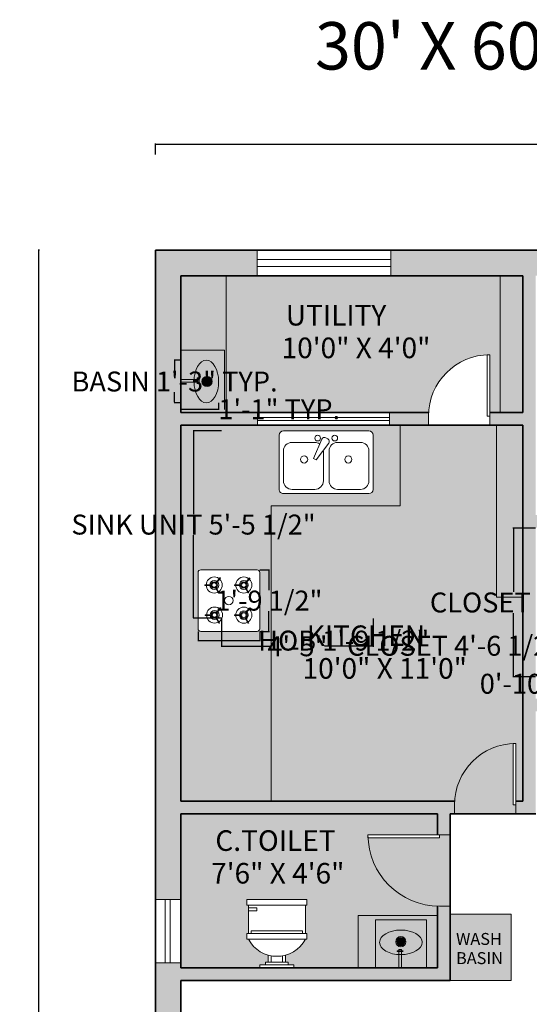
# Model space of a CAD drawing. Units: inches. Extents: x 2167 to 2589, y 1680 to 2489.
# Tile 35 of 38: x 2167 to 2346, y 2143 to 2489. Entities that reach past the tile are written whole.
import ezdxf

# ---------------------------------------------------------------- set-up
doc = ezdxf.new("R2010")
doc.units = ezdxf.units.IN
doc.header["$MEASUREMENT"] = 0
doc.layers.get('0').update_dxf_attribs({"color": 250})
for name, color, linetype, lineweight in [('A-ANNO-DIMS', 2, 'Continuous', 18), ('A-AREA-IDEN', 7, 'Continuous', 18), ('A-DOOR', 4, 'Continuous', 18), ('A-EQPM', 34, 'Continuous', 18), ('A-FLOR-FIXT', 8, 'Continuous', 18), ('A-FURN-FIXD', 34, 'Continuous', 18), ('A-WALL-PATT', 250, 'Continuous', 13), ('C-PROP', 7, 'Continuous', 35), ('furniture', 34, 'Continuous', 18), ('text', 7, 'Continuous', 25), ('walls', 7, 'Continuous', 35), ('windows', 141, 'Continuous', 18)]:
    doc.layers.add(name, color=color, linetype=linetype, lineweight=lineweight)
for name, color, linetype, lineweight, true_color in [('A-FLOR-FIXT-PATT', 7, 'Continuous', 13, 0xebebeb), ('A-FLOR-PATT', 254, 'Continuous', 13, 0xfeeab9), ('A-FURN-FIXD-PATT', 33, 'Continuous', 13, 0xcd8e5c)]:
    doc.layers.add(name, color=color, linetype=linetype, lineweight=lineweight, true_color=true_color)
doc.styles.add('ATT', font='TXT')
doc.styles.get("Standard").update_dxf_attribs({"font": 'arial.ttf'})
doc.dimstyles.get("Standard").update_dxf_attribs({"dimtxt": 7, "dimasz": 0.18, "dimexe": 0.18, "dimexo": 0.0625, "dimgap": 0.09, "dimtad": 0, "dimtih": 1, "dimtoh": 1, "dimdec": 1, "dimzin": 0, "dimdsep": 46, "dimlunit": 3, "dimtxsty": 'Standard', "dimcen": 0.09, "dimadec": 0, "dimazin": 0, "dimtfac": 1, "dimtdec": 1, "dimtofl": 0, "dimtmove": 0, "dimatfit": 3, "dimfxl": 1, "dimtolj": 1, "dimtzin": 0, "dimarcsym": 0})

# ---------------------------------------------------------------- blocks, each defined once
blk = doc.blocks.new('*U2')
for p, q in [((0, 0), (0, -6)), ((40, 0), (40, -6))]:
    blk.add_line(p, q)
blk.add_lwpolyline([(0, 0), (0, 40), (1.75, 40), (1.75, 0)], close=True)
blk.add_arc((0, 0), 40, 0, 90)
blk = doc.blocks.new('4bstove')
at = {"layer": 'furniture'}
for p, q in [((1452.73, 1446.21), (1452.73, 1448.61)), ((1452.98, 1446.22), (1452.98, 1448.61)), ((1464.44, 1446.34), (1464.44, 1448.73)), ((1464.69, 1446.34), (1464.69, 1448.73)), ((1463.45, 1444.58), (1461.38, 1443.38)), ((1451.74, 1444.45), (1449.67, 1443.25)), ((1451.87, 1444.23), (1449.79, 1443.04)), ((1453.75, 1444.08), (1455.58, 1442.54)), ((1453.91, 1444.27), (1455.74, 1442.73)), ((1463.57, 1444.36), (1461.5, 1443.17)), ((1465.46, 1444.21), (1467.29, 1442.67)), ((1465.62, 1444.4), (1467.45, 1442.86)), ((1452.69, 1434.81), (1452.69, 1437.2)), ((1452.94, 1434.81), (1452.94, 1437.2)), ((1464.44, 1434.81), (1464.44, 1437.2)), ((1464.69, 1434.81), (1464.69, 1437.2)), ((1451.7, 1433.04), (1449.63, 1431.85)), ((1463.45, 1433.04), (1461.38, 1431.85)), ((1451.82, 1432.83), (1449.75, 1431.63)), ((1453.71, 1432.67), (1455.54, 1431.13)), ((1453.87, 1432.86), (1455.7, 1431.33)), ((1463.57, 1432.83), (1461.5, 1431.63)), ((1465.46, 1432.67), (1467.29, 1431.13)), ((1465.62, 1432.86), (1467.45, 1431.33))]:
    blk.add_line(p, q, dxfattribs=at)
for points in [[(1447.5, 1427.38), (1469.5, 1427.38, 0.414214), (1470.5, 1428.38), (1470.5, 1450.38, 0.414214), (1469.5, 1451.38), (1447.5, 1451.38, 0.414214), (1446.5, 1450.38), (1446.5, 1428.38, 0.414214)], [(1453.75, 1444.97, 1), (1452, 1444.97, 1)], [(1465.46, 1445.1, 1), (1463.71, 1445.1, 1)], [(1453.71, 1433.56, 1), (1451.96, 1433.56, 1)], [(1465.46, 1433.56, 1), (1463.71, 1433.56, 1)]]:
    blk.add_lwpolyline(points, format="xyb", close=True, dxfattribs=at)
for points in [[(1454.12, 1444.97, 1), (1451.62, 1444.97, 1), (1454.12, 1444.97, 1)], [(1465.83, 1445.1, 1), (1463.33, 1445.1, 1), (1465.83, 1445.1, 1)], [(1454.08, 1433.56, 1), (1451.58, 1433.56, 1), (1454.08, 1433.56, 1)], [(1465.83, 1433.56, 1), (1463.33, 1433.56, 1), (1465.83, 1433.56, 1)]]:
    blk.add_lwpolyline(points, format="xyb", dxfattribs=at)
for centre, radius in [((1452.87, 1444.97), 3.14), ((1452.87, 1444.97), 1.75), ((1464.58, 1445.1), 3.14), ((1464.58, 1445.1), 1.75), ((1458.5, 1439.38), 1.67), ((1452.83, 1433.56), 3.14), ((1452.83, 1433.56), 1.75), ((1464.58, 1433.56), 3.14), ((1464.58, 1433.56), 1.75)]:
    blk.add_circle(centre, radius, dxfattribs=at)
for centre, start, end in [((1452.87, 1444.97), 88.2645, 92.2039), ((1464.58, 1445.1), 88.2645, 92.2039), ((1452.87, 1444.97), 208.188, 212.1274), ((1452.87, 1444.97), 318.1018, 322.0412), ((1464.58, 1445.1), 208.188, 212.1274), ((1464.58, 1445.1), 318.1018, 322.0412), ((1452.83, 1433.56), 88.2645, 92.2039), ((1464.58, 1433.56), 88.2645, 92.2039)]:
    blk.add_arc(centre, 3.64, start, end, dxfattribs=at)
blk = doc.blocks.new('stove')
at = {"layer": 'furniture', "xscale": 0.9, "yscale": 0.9, "zscale": 0.9, "rotation": 89.99999999999999}
blk.add_blockref('4bstove', (1295.44, -1312.65), dxfattribs=at)
blk = doc.blocks.new('15PSNK10')
at = {"color": 0, "linetype": 'ByBlock'}
for p, q in [((0, 15), (0, -15)), ((20.5, 16.5), (1.5, 16.5)), ((7, 15), (17.5, 15)), ((22, -15), (22, 15)), ((4, 4), (4, 12)), ((20.5, 12), (20.5, 4)), ((2.37, -0.1), (2.77, 0.6)), ((10.18, -3.57), (4.27, 0.87)), ((17.5, 1), (7, 1)), ((2.88, -1.54), (9.68, -4.43)), ((7.04, -1), (17.5, -1)), ((4, -12), (4, -4)), ((9.68, -4.43), (10.18, -3.57)), ((20.5, -4), (20.5, -12)), ((1.5, -16.5), (20.5, -16.5)), ((17.5, -15), (7, -15))]:
    blk.add_line(p, q, dxfattribs=at)
for centre, radius in [((10, 7.75), 1.25), ((2.5, 3), 1), ((2.5, -3), 1), ((10, -7.75), 1.25)]:
    blk.add_circle(centre, radius, dxfattribs=at)
for centre, radius, start, end in [((1.5, 15), 1.5, 90, 180), ((7, 12), 3, 90, 180), ((17.5, 12), 3, 0, 90), ((20.5, 15), 1.5, 0, 90), ((7, 4), 3, 180, 270), ((17.5, 4), 3, 270, 0), ((3.63, 0.1), 1, 50.5377, 150), ((3.23, -0.6), 1, 150, 249.4623), ((7, -4), 3, 146.607, 180), ((17.5, -4), 3, 0, 90), ((7, -12), 3, 180, 270), ((17.5, -12), 3, 270, 0), ((1.5, -15), 1.5, 180, 270), ((20.5, -15), 1.5, 270, 0)]:
    blk.add_arc(centre, radius, start, end, dxfattribs=at)
at = {"color": 0, "linetype": 'ByBlock', "style": 'ATT'}
for tag, p, flags in [('ITEM', (0, -26), 3), ('ROOM_NUMBER', (0, -35), 1)]:
    blk.add_attdef(tag, p, '', height=6, dxfattribs=dict(at, flags=flags))
blk = doc.blocks.new('*U11')
for p, q in [((-10, 22), (-10, 12)), ((-10, 21), (-7, 21)), ((-7, 21), (-7, 20)), ((10, 12), (10, 22)), ((-7, 20), (-10, 20)), ((10.5, 12), (-10.5, 12)), ((-10.5, 10), (-10.5, 12)), ((9, 13), (-9, 13)), ((-9, 13), (-9, 12)), ((9, 12), (9, 13)), ((10.5, 12), (10.5, 10)), ((10.5, 10), (-10.5, 10)), ((-3, 4.4065), (-3, 2)), ((-2, 2), (-2, 4.1658)), ((2, 4.1658), (2, 2)), ((3, 2), (3, 4.4065)), ((4, 2), (-4, 2)), ((-4, 2), (-4, 1)), ((4, 1), (4, 2))]:
    blk.add_line(p, q)
for points in [[(10.5, 22), (10.5, 24), (-10.5, 24), (-10.5, 22)], [(6, 0), (6, 1), (-6, 1), (-6, 0)]]:
    blk.add_lwpolyline(points, close=True)
blk.add_arc((0, 15.3333), 11.3333, 208.0725, 331.9275)
blk = doc.blocks.new('*D23')
at = {"layer": 'A-ANNO-DIMS', "color": 0, "lineweight": -2, "transparency": 16777216}
for p, q in [((2215.05, 2441.31), (2215.05, 2445.11)), ((2215.23, 2444.93), (2389.02, 2444.93)), ((2574.87, 2444.93), (2401.08, 2444.93)), ((2575.05, 2441.31), (2575.05, 2445.11))]:
    blk.add_line(p, q, dxfattribs=at)
at = {"layer": 'A-ANNO-DIMS', "color": 0, "transparency": 16777216}
for points in [[(2215.23, 2444.96), (2215.23, 2444.9), (2215.05, 2444.93)], [(2574.87, 2444.96), (2574.87, 2444.9), (2575.05, 2444.93)]]:
    blk.add_solid(points, dxfattribs=at)
at = {"layer": 'Defpoints', "color": 0, "transparency": 16777216}
for p in [(2575.05, 2444.93), (2215.05, 2441.25), (2575.05, 2441.25)]:
    blk.add_point(p, dxfattribs=at)
at = {"layer": 'A-ANNO-DIMS', "color": 0, "transparency": 16777216, "insert": (2395.05, 2444.93), "char_height": 7, "attachment_point": 5}
blk.add_mtext("\\A1;30'", dxfattribs=at)
blk = doc.blocks.new('*D24')
at = {"layer": 'A-ANNO-DIMS', "color": 0, "lineweight": -2, "transparency": 16777216}
for p, q in [((2174.43, 2407.69), (2173.89, 2407.69)), ((2174.07, 2407.51), (2174.07, 2051.36)), ((2174.07, 1687.87), (2174.07, 2044.03)), ((2174.43, 1687.69), (2173.89, 1687.69))]:
    blk.add_line(p, q, dxfattribs=at)
at = {"layer": 'A-ANNO-DIMS', "color": 0, "transparency": 16777216}
for points in [[(2174.04, 2407.51), (2174.1, 2407.51), (2174.07, 2407.69)], [(2174.04, 1687.87), (2174.1, 1687.87), (2174.07, 1687.69)]]:
    blk.add_solid(points, dxfattribs=at)
at = {"layer": 'Defpoints', "color": 0, "transparency": 16777216}
for p in [(2174.49, 2407.69), (2174.07, 1687.69), (2174.49, 1687.69)]:
    blk.add_point(p, dxfattribs=at)
at = {"layer": 'A-ANNO-DIMS', "color": 0, "transparency": 16777216, "insert": (2174.07, 2047.69), "char_height": 7, "attachment_point": 5}
blk.add_mtext("\\A1;60'", dxfattribs=at)
blk = doc.blocks.new('LAV-OVAL-WITH-TAP')
for p, q in [((6.14, 5.63), (6.14, 5.92)), ((6.14, 5.92), (8.26, 5.92)), ((8.26, 5.63), (6.14, 5.63)), ((7.69, 6.42), (6.74, 6.42)), ((6.74, 6.42), (6.74, 0)), ((7.69, 6.42), (7.69, 0))]:
    blk.add_line(p, q)
for radius in [1.79, 1.79, 1.43, 1.43, 1.43, 1.43]:
    blk.add_circle((7.46, 9.13), radius)
blk.add_ellipse((7.48, 8.9), major_axis=(7.48, 0.02), ratio=0.576535)
blk = doc.blocks.new('*D31')
at = {"layer": 'A-ANNO-DIMS', "color": 0, "lineweight": -2, "transparency": 16777216}
for p, q in [((2223.99, 2369.03), (2221.62, 2369.03)), ((2221.8, 2368.85), (2221.8, 2365.26)), ((2221.8, 2354.24), (2221.8, 2357.83)), ((2223.99, 2354.06), (2221.62, 2354.06))]:
    blk.add_line(p, q, dxfattribs=at)
at = {"layer": 'A-ANNO-DIMS', "color": 0, "transparency": 16777216}
for points in [[(2221.77, 2368.85), (2221.83, 2368.85), (2221.8, 2369.03)], [(2221.77, 2354.24), (2221.83, 2354.24), (2221.8, 2354.06)]]:
    blk.add_solid(points, dxfattribs=at)
at = {"layer": 'Defpoints', "color": 0, "transparency": 16777216}
for p in [(2224.05, 2369.03), (2221.8, 2354.06), (2224.05, 2354.06)]:
    blk.add_point(p, dxfattribs=at)
at = {"layer": 'A-ANNO-DIMS', "color": 0, "transparency": 16777216, "insert": (2221.8, 2361.54), "char_height": 7, "attachment_point": 5}
blk.add_mtext('\\A1;BASIN 1\'-3" TYP.', dxfattribs=at)
blk = doc.blocks.new('*D32')
at = {"layer": 'A-ANNO-DIMS', "color": 0, "lineweight": -2, "transparency": 16777216}
for p, q in [((2224.05, 2354), (2224.05, 2351.63)), ((2224.23, 2351.81), (2237.09, 2351.81)), ((2237.27, 2354), (2237.27, 2351.63)), ((2237.27, 2351.81), (2237.45, 2351.81))]:
    blk.add_line(p, q, dxfattribs=at)
at = {"layer": 'A-ANNO-DIMS', "color": 0, "transparency": 16777216}
for points in [[(2224.23, 2351.84), (2224.23, 2351.78), (2224.05, 2351.81)], [(2237.09, 2351.84), (2237.09, 2351.78), (2237.27, 2351.81)]]:
    blk.add_solid(points, dxfattribs=at)
at = {"layer": 'Defpoints', "color": 0, "transparency": 16777216}
for p in [(2224.05, 2354.06), (2237.27, 2354.06), (2237.27, 2351.81)]:
    blk.add_point(p, dxfattribs=at)
at = {"layer": 'A-ANNO-DIMS', "color": 0, "transparency": 16777216, "insert": (2258.54, 2351.81), "char_height": 7, "attachment_point": 5}
blk.add_mtext('\\A1;1\'-1" TYP.', dxfattribs=at)
blk = doc.blocks.new('*D33')
at = {"layer": 'A-ANNO-DIMS', "color": 0, "lineweight": -2, "transparency": 16777216}
for p, q in [((2358.53, 2268.74), (2358.35, 2268.74)), ((2358.53, 2260.62), (2358.53, 2268.92)), ((2412.91, 2268.74), (2358.71, 2268.74)), ((2413.09, 2260.62), (2413.09, 2268.92))]:
    blk.add_line(p, q, dxfattribs=at)
at = {"layer": 'A-ANNO-DIMS', "color": 0, "transparency": 16777216}
for points in [[(2358.71, 2268.77), (2358.71, 2268.71), (2358.53, 2268.74)], [(2412.91, 2268.77), (2412.91, 2268.71), (2413.09, 2268.74)]]:
    blk.add_solid(points, dxfattribs=at)
at = {"layer": 'Defpoints', "color": 0, "transparency": 16777216}
for p in [(2358.53, 2268.74), (2358.53, 2260.56), (2413.09, 2260.56)]:
    blk.add_point(p, dxfattribs=at)
at = {"layer": 'A-ANNO-DIMS', "color": 0, "transparency": 16777216, "insert": (2319.92, 2268.74), "char_height": 7, "attachment_point": 5}
blk.add_mtext('\\A1;CLOSET 4\'-6 1/2"', dxfattribs=at)
blk = doc.blocks.new('*D34')
at = {"layer": 'A-ANNO-DIMS', "color": 0, "lineweight": -2, "transparency": 16777216}
for p, q in [((2358.47, 2260.56), (2350.17, 2260.56)), ((2350.35, 2260.38), (2350.35, 2259.11)), ((2350.35, 2250.42), (2350.35, 2251.69)), ((2358.47, 2250.24), (2350.17, 2250.24))]:
    blk.add_line(p, q, dxfattribs=at)
at = {"layer": 'A-ANNO-DIMS', "color": 0, "transparency": 16777216}
for points in [[(2350.32, 2260.38), (2350.38, 2260.38), (2350.35, 2260.56)], [(2350.32, 2250.42), (2350.38, 2250.42), (2350.35, 2250.24)]]:
    blk.add_solid(points, dxfattribs=at)
at = {"layer": 'Defpoints', "color": 0, "transparency": 16777216}
for p in [(2358.53, 2260.56), (2350.35, 2250.24), (2358.53, 2250.24)]:
    blk.add_point(p, dxfattribs=at)
at = {"layer": 'A-ANNO-DIMS', "color": 0, "transparency": 16777216, "insert": (2350.35, 2255.4), "char_height": 7, "attachment_point": 5}
blk.add_mtext('\\A1;0\'-10 1/2"', dxfattribs=at)
blk = doc.blocks.new('*D37')
at = {"layer": 'A-ANNO-DIMS', "color": 0, "lineweight": -2, "transparency": 16777216}
for p, q in [((2348.49, 2310.05), (2340.54, 2310.05)), ((2340.72, 2309.87), (2340.72, 2287.66)), ((2340.72, 2258.02), (2340.72, 2280.23)), ((2348.49, 2257.84), (2340.54, 2257.84))]:
    blk.add_line(p, q, dxfattribs=at)
at = {"layer": 'A-ANNO-DIMS', "color": 0, "transparency": 16777216}
for points in [[(2340.69, 2309.87), (2340.75, 2309.87), (2340.72, 2310.05)], [(2340.69, 2258.02), (2340.75, 2258.02), (2340.72, 2257.84)]]:
    blk.add_solid(points, dxfattribs=at)
at = {"layer": 'Defpoints', "color": 0, "transparency": 16777216}
for p in [(2348.55, 2310.05), (2340.72, 2257.84), (2348.55, 2257.84)]:
    blk.add_point(p, dxfattribs=at)
at = {"layer": 'A-ANNO-DIMS', "color": 0, "transparency": 16777216, "insert": (2340.72, 2283.95), "char_height": 7, "attachment_point": 5}
blk.add_mtext('\\A1;CLOSET 4\'-4"', dxfattribs=at)
blk = doc.blocks.new('*D49')
at = {"layer": 'A-ANNO-DIMS', "color": 0, "lineweight": -2, "transparency": 16777216}
for p, q in [((2230.07, 2273.74), (2230.07, 2270.38)), ((2251.67, 2273.74), (2251.67, 2270.38)), ((2230.25, 2270.56), (2251.49, 2270.56)), ((2251.67, 2270.56), (2251.85, 2270.56))]:
    blk.add_line(p, q, dxfattribs=at)
at = {"layer": 'A-ANNO-DIMS', "color": 0, "transparency": 16777216}
for points in [[(2230.25, 2270.59), (2230.25, 2270.53), (2230.07, 2270.56)], [(2251.49, 2270.59), (2251.49, 2270.53), (2251.67, 2270.56)]]:
    blk.add_solid(points, dxfattribs=at)
at = {"layer": 'Defpoints', "color": 0, "transparency": 16777216}
for p in [(2230.07, 2273.8), (2251.67, 2273.8), (2251.67, 2270.56)]:
    blk.add_point(p, dxfattribs=at)
at = {"layer": 'A-ANNO-DIMS', "color": 0, "transparency": 16777216, "insert": (2281.17, 2270.56), "char_height": 7, "attachment_point": 5}
blk.add_mtext('\\A1;HOB 1\'-9 1/2"', dxfattribs=at)
blk = doc.blocks.new('*D50')
at = {"layer": 'A-ANNO-DIMS', "color": 0, "lineweight": -2, "transparency": 16777216}
for p, q in [((2251.74, 2295.4), (2255.09, 2295.4)), ((2254.91, 2295.22), (2254.91, 2288.31)), ((2254.91, 2273.98), (2254.91, 2280.89)), ((2251.74, 2273.8), (2255.09, 2273.8))]:
    blk.add_line(p, q, dxfattribs=at)
at = {"layer": 'A-ANNO-DIMS', "color": 0, "transparency": 16777216}
for points in [[(2254.88, 2295.22), (2254.94, 2295.22), (2254.91, 2295.4)], [(2254.88, 2273.98), (2254.94, 2273.98), (2254.91, 2273.8)]]:
    blk.add_solid(points, dxfattribs=at)
at = {"layer": 'Defpoints', "color": 0, "transparency": 16777216}
for p in [(2251.67, 2295.4), (2254.91, 2295.4), (2251.67, 2273.8)]:
    blk.add_point(p, dxfattribs=at)
at = {"layer": 'A-ANNO-DIMS', "color": 0, "transparency": 16777216, "insert": (2254.91, 2284.6), "char_height": 7, "attachment_point": 5}
blk.add_mtext('\\A1;1\'-9 1/2"', dxfattribs=at)
blk = doc.blocks.new('*D53')
at = {"layer": 'A-ANNO-DIMS', "color": 0, "lineweight": -2, "transparency": 16777216}
for p, q in [((2238.25, 2344.17), (2228.27, 2344.17)), ((2228.45, 2343.99), (2228.45, 2315.01)), ((2228.45, 2278.61), (2228.45, 2307.59)), ((2238.25, 2278.43), (2228.27, 2278.43))]:
    blk.add_line(p, q, dxfattribs=at)
at = {"layer": 'A-ANNO-DIMS', "color": 0, "transparency": 16777216}
for points in [[(2228.42, 2343.99), (2228.48, 2343.99), (2228.45, 2344.17)], [(2228.42, 2278.61), (2228.48, 2278.61), (2228.45, 2278.43)]]:
    blk.add_solid(points, dxfattribs=at)
at = {"layer": 'Defpoints', "color": 0, "transparency": 16777216}
for p in [(2238.31, 2344.17), (2228.45, 2278.43), (2238.31, 2278.43)]:
    blk.add_point(p, dxfattribs=at)
at = {"layer": 'A-ANNO-DIMS', "color": 0, "transparency": 16777216, "insert": (2228.45, 2311.3), "char_height": 7, "attachment_point": 5}
blk.add_mtext('\\A1;SINK UNIT 5\'-5 1/2"', dxfattribs=at)
blk = doc.blocks.new('*D54')
at = {"layer": 'A-ANNO-DIMS', "color": 0, "lineweight": -2, "transparency": 16777216}
for p, q in [((2238.31, 2278.36), (2238.31, 2268.39)), ((2291.52, 2278.36), (2291.52, 2268.39)), ((2238.49, 2268.57), (2255.38, 2268.57)), ((2291.34, 2268.57), (2274.45, 2268.57))]:
    blk.add_line(p, q, dxfattribs=at)
at = {"layer": 'A-ANNO-DIMS', "color": 0, "transparency": 16777216}
for points in [[(2238.49, 2268.6), (2238.49, 2268.54), (2238.31, 2268.57)], [(2291.34, 2268.6), (2291.34, 2268.54), (2291.52, 2268.57)]]:
    blk.add_solid(points, dxfattribs=at)
at = {"layer": 'Defpoints', "color": 0, "transparency": 16777216}
for p in [(2238.31, 2278.43), (2291.52, 2278.43), (2291.52, 2268.57)]:
    blk.add_point(p, dxfattribs=at)
at = {"layer": 'A-ANNO-DIMS', "color": 0, "transparency": 16777216, "insert": (2264.92, 2268.57), "char_height": 7, "attachment_point": 5}
blk.add_mtext('\\A1;4\'-5"', dxfattribs=at)

msp = doc.modelspace()

# ---------------------------------------------------------------- hatches: boundary and pattern name
at = {"layer": 'A-FLOR-FIXT-PATT'}
h = msp.add_hatch(color=256, dxfattribs=at)
h.dxf.hatch_style = 1
edge = h.paths.add_edge_path()
edge.add_line((2239.3, 2351.68), (2239.3, 2372.58))
edge.add_line((2239.3, 2372.58), (2224.05, 2372.58))
edge.add_line((2224.05, 2372.58), (2224.05, 2362.28))
edge.add_line((2224.05, 2362.28), (2228.65, 2362.28))
edge.add_ellipse((2232.94, 2361.54), major_axis=(0.02, -7.48), ratio=0.576535, start_angle=272.6137, end_angle=620.1108, ccw=False)
edge.add_line((2228.63, 2361.34), (2224.05, 2361.34))
edge.add_line((2224.05, 2361.34), (2224.05, 2351.68))
edge.add_line((2224.05, 2351.68), (2239.3, 2351.68))
h = msp.add_hatch(color=256, dxfattribs=at)
h.dxf.hatch_style = 1
edge = h.paths.add_edge_path()
edge.add_ellipse((2232.94, 2361.54), major_axis=(0.02, -7.48), ratio=0.576535, start_angle=272.6137, end_angle=260.1108)
edge.add_line((2228.65, 2362.28), (2229.68, 2362.28))
edge.add_line((2229.68, 2362.28), (2229.68, 2362.88))
edge.add_line((2229.68, 2362.88), (2229.97, 2362.88))
edge.add_line((2229.97, 2362.88), (2229.97, 2362.28))
edge.add_line((2229.97, 2362.28), (2230.47, 2362.28))
edge.add_line((2230.47, 2362.28), (2230.47, 2361.34))
edge.add_line((2230.47, 2361.34), (2228.63, 2361.34))
h.paths.add_polyline_path([(2233.18, 2359.77, -1), (2233.18, 2363.35, -1)], flags=16)
h.paths.add_polyline_path([(2233.18, 2362.99, -1), (2233.18, 2360.13, -1)], flags=0)
h.paths.add_polyline_path([(2233.18, 2360.13, 1), (2233.18, 2362.99, 1)], flags=0)
edge = h.paths.add_edge_path()
edge.add_line((2229.68, 2361.34), (2229.68, 2362.28))
edge.add_line((2229.68, 2362.28), (2228.65, 2362.28))
edge.add_ellipse((2232.94, 2361.54), major_axis=(0.02, -7.48), ratio=0.576535, start_angle=260.1108, end_angle=272.6137)
edge.add_line((2228.63, 2361.34), (2229.68, 2361.34))
h.paths.add_polyline_path([(2230.47, 2361.34), (2230.47, 2362.28), (2229.97, 2362.28), (2229.97, 2361.34)], flags=17)
h.paths.add_polyline_path([(2229.97, 2361.34), (2229.97, 2362.28), (2229.68, 2362.28), (2229.68, 2361.34)], flags=17)
h.paths.add_polyline_path([(2229.97, 2362.28), (2229.97, 2362.88), (2229.68, 2362.88), (2229.68, 2362.28)], flags=17)
edge = h.paths.add_edge_path()
edge.add_ellipse((2232.94, 2361.54), major_axis=(0.02, -7.48), ratio=0.576535, start_angle=260.1108, end_angle=272.6137, ccw=False)
edge.add_line((2228.65, 2362.28), (2224.05, 2362.28))
edge.add_line((2224.05, 2362.28), (2224.05, 2361.34))
edge.add_line((2224.05, 2361.34), (2228.63, 2361.34))
h = msp.add_hatch(color=256, dxfattribs=at)
h.dxf.hatch_style = 1
h.paths.add_polyline_path([(2233.18, 2362.99, 1), (2233.18, 2360.13, 1)], flags=0)
h.paths.add_polyline_path([(2233.18, 2363.35, 1), (2233.18, 2359.77, 1)])
h.paths.add_polyline_path([(2233.18, 2362.99, -1), (2233.18, 2360.13, -1)], flags=16)
h = msp.add_hatch(color=256, dxfattribs=at)
h.dxf.hatch_style = 1
h.paths.add_polyline_path([(2233.18, 2362.99, 1), (2233.18, 2360.13, 1)])
h = msp.add_hatch(color=256, dxfattribs=at)
h.dxf.hatch_style = 1
edge = h.paths.add_edge_path()
edge.add_line((2310.18, 2172.5), (2292.31, 2172.5))
edge.add_line((2292.31, 2172.5), (2292.31, 2155.69))
edge.add_line((2292.31, 2155.69), (2300.49, 2155.69))
edge.add_line((2300.49, 2155.69), (2300.49, 2160.3))
edge.add_ellipse((2301.23, 2164.59), major_axis=(7.48, 0.02), ratio=0.576535, start_angle=272.6137, end_angle=620.1108, ccw=False)
edge.add_line((2301.44, 2160.28), (2301.44, 2155.69))
edge.add_line((2301.44, 2155.69), (2310.18, 2155.69))
edge.add_line((2310.18, 2155.69), (2310.18, 2172.5))
h = msp.add_hatch(color=256, dxfattribs=at)
h.dxf.hatch_style = 1
edge = h.paths.add_edge_path()
edge.add_ellipse((2301.23, 2164.59), major_axis=(7.48, 0.02), ratio=0.576535, start_angle=272.6137, end_angle=260.1108)
edge.add_line((2300.49, 2160.3), (2300.49, 2161.32))
edge.add_line((2300.49, 2161.32), (2299.89, 2161.32))
edge.add_line((2299.89, 2161.32), (2299.89, 2161.62))
edge.add_line((2299.89, 2161.62), (2300.49, 2161.62))
edge.add_line((2300.49, 2161.62), (2300.49, 2162.11))
edge.add_line((2300.49, 2162.11), (2301.44, 2162.11))
edge.add_line((2301.44, 2162.11), (2301.44, 2160.28))
h.paths.add_polyline_path([(2303, 2164.83, -1), (2299.43, 2164.83, -1)], flags=16)
h.paths.add_polyline_path([(2299.79, 2164.83, -1), (2302.64, 2164.83, -1)], flags=0)
edge = h.paths.add_edge_path()
edge.add_ellipse((2301.23, 2164.59), major_axis=(7.48, 0.02), ratio=0.576535, start_angle=260.1108, end_angle=272.6137, ccw=False)
edge.add_line((2300.49, 2160.3), (2300.49, 2155.69))
edge.add_line((2300.49, 2155.69), (2301.44, 2155.69))
edge.add_line((2301.44, 2155.69), (2301.44, 2160.28))
edge = h.paths.add_edge_path()
edge.add_line((2301.44, 2161.32), (2300.49, 2161.32))
edge.add_line((2300.49, 2161.32), (2300.49, 2160.3))
edge.add_ellipse((2301.23, 2164.59), major_axis=(7.48, 0.02), ratio=0.576535, start_angle=260.1108, end_angle=272.6137)
edge.add_line((2301.44, 2160.28), (2301.44, 2161.32))
h.paths.add_polyline_path([(2301.44, 2162.11), (2300.49, 2162.11), (2300.49, 2161.62), (2301.44, 2161.62)], flags=17)
h.paths.add_polyline_path([(2301.44, 2161.62), (2300.49, 2161.62), (2300.49, 2161.32), (2301.44, 2161.32)], flags=17)
h.paths.add_polyline_path([(2300.49, 2161.62), (2299.89, 2161.62), (2299.89, 2161.32), (2300.49, 2161.32)], flags=17)
h = msp.add_hatch(color=256, dxfattribs=at)
h.dxf.hatch_style = 1
h.paths.add_polyline_path([(2302.64, 2164.83, 1), (2299.79, 2164.83, 1)])
at = {"layer": 'A-FLOR-PATT'}
h = msp.add_hatch(color=256, dxfattribs=at)
h.dxf.hatch_style = 1
h.paths.add_polyline_path([(2331.51, 2370.93), (2331.51, 2370.95), (2332.45, 2370.95), (2332.45, 2350.69), (2336.06, 2350.69), (2336.06, 2398.69), (2239.96, 2398.69), (2239.96, 2373.2), (2239.96, 2350.69), (2310.96, 2350.69, -0.38441)])
h = msp.add_hatch(color=256, dxfattribs=at)
h.dxf.hatch_style = 1
h.paths.add_polyline_path([(2289.71, 2201.31), (2289.68, 2201.31), (2289.68, 2202.4), (2314.05, 2202.4), (2314.05, 2209.69), (2224.05, 2209.69), (2224.05, 2155.69), (2251.7, 2155.69), (2251.7, 2156.69), (2253.7, 2156.69), (2253.7, 2157.69), (2254.7, 2157.69), (2254.7, 2160.1, -0.206081), (2247.7, 2165.69), (2247.2, 2165.69), (2247.2, 2167.69), (2247.7, 2167.69), (2247.7, 2177.69), (2247.2, 2177.69), (2247.2, 2179.69), (2268.2, 2179.69), (2268.2, 2177.69), (2267.7, 2177.69), (2267.7, 2167.69), (2268.2, 2167.69), (2268.2, 2165.69), (2267.7, 2165.69, -0.206081), (2260.7, 2160.1), (2260.7, 2157.69), (2261.7, 2157.69), (2261.7, 2156.69), (2263.7, 2156.69), (2263.7, 2155.69), (2286.21, 2155.69), (2286.21, 2173.97), (2314.05, 2173.97), (2314.05, 2177.32, -0.392973)])
h.paths.add_polyline_path([(2318.55, 2202.4), (2314.78, 2202.4), (2314.78, 2201.31), (2289.71, 2201.31, 0.401453), (2314.78, 2177.3), (2318.55, 2177.3)])
h.paths.add_polyline_path([(2344.05, 2285.87), (2334.79, 2285.87), (2334.79, 2346.19), (2300.97, 2346.19), (2300.97, 2317.9), (2255.65, 2317.9), (2255.65, 2214.19), (2320.1, 2214.19, -0.38441), (2340.65, 2234.43), (2340.65, 2234.45), (2341.59, 2234.45), (2341.59, 2214.19), (2344.05, 2214.19)])
h.paths.add_polyline_path([(2340.65, 2234.43, 0.401453), (2320.06, 2212.92), (2320.06, 2209.69), (2341.59, 2209.69), (2341.59, 2212.92), (2340.65, 2212.92)])
at = {"layer": 'A-FURN-FIXD-PATT'}
h = msp.add_hatch(color=256, dxfattribs=at)
h.dxf.hatch_style = 1
h.paths.add_polyline_path([(2239.96, 2398.69), (2224.05, 2398.69), (2224.05, 2373.2), (2239.96, 2373.2)])
h = msp.add_hatch(color=256, dxfattribs=at)
h.dxf.hatch_style = 1
h.paths.add_polyline_path([(2344.05, 2398.69), (2336.06, 2398.69), (2336.06, 2350.69), (2344.05, 2350.69)])
h = msp.add_hatch(color=256, dxfattribs=at)
h.dxf.hatch_style = 1
h.paths.add_polyline_path([(2239.96, 2351.05), (2239.96, 2373.2), (2224.05, 2373.2), (2224.05, 2372.58), (2239.3, 2372.58), (2239.3, 2351.68), (2224.05, 2351.68), (2224.05, 2351.05)])
h = msp.add_hatch(color=256, dxfattribs=at)
h.dxf.hatch_style = 1
h.paths.add_polyline_path([(2300.97, 2346.19), (2224.05, 2346.19), (2224.05, 2214.19), (2255.65, 2214.19), (2255.65, 2317.9), (2300.97, 2317.9)])
h.paths.add_polyline_path([(2260.02, 2322.17, -0.414214), (2258.52, 2323.67), (2258.52, 2342.67, -0.414214), (2260.02, 2344.17), (2290.02, 2344.17, -0.414214), (2291.52, 2342.67), (2291.52, 2323.67, -0.414214), (2290.02, 2322.17)], flags=16)
h.paths.add_polyline_path([(2276.02, 2326.67), (2276.02, 2337.17, -0.414214), (2279.02, 2340.17), (2287.02, 2340.17, -0.414214), (2290.02, 2337.17), (2290.02, 2326.67, -0.414214), (2287.02, 2323.67), (2279.02, 2323.67, -0.414214)], flags=0)
h.paths.add_polyline_path([(2266.02, 2334.17, -1), (2268.52, 2334.17, -1)], flags=0)
h.paths.add_polyline_path([(2271.46, 2333.99), (2270.59, 2334.49), (2273.49, 2341.28, -0.463199), (2274.92, 2341.8), (2275.62, 2341.4, -0.463705), (2275.89, 2339.9)], flags=0)
h.paths.add_polyline_path([(2281.52, 2334.17, -1), (2284.02, 2334.17, -1)], flags=0)
h.paths.add_polyline_path([(2271.02, 2341.67, -1), (2273.02, 2341.67, -1)], flags=0)
h.paths.add_polyline_path([(2277.02, 2341.67, -1), (2279.02, 2341.67, -1)], flags=0)
h.paths.add_polyline_path([(2251.67, 2294.5), (2251.67, 2274.7, -0.414214), (2250.77, 2273.8), (2230.97, 2273.8, -0.414214), (2230.07, 2274.7), (2230.07, 2294.5, -0.414214), (2230.97, 2295.4), (2250.77, 2295.4, -0.414214)], flags=16)
h.paths.add_polyline_path([(2248.93, 2290.07, -0.977944), (2243.29, 2289.95), (2242.84, 2289.95, -0.017191), (2242.84, 2290.17), (2243.29, 2290.17, -0.982592)], flags=0)
h.paths.add_polyline_path([(2247.68, 2290.07, -1), (2244.53, 2290.07, -1)], flags=0)
h.paths.add_polyline_path([(2246.11, 2288.95, -1), (2246.11, 2291.2, -1)], flags=0)
h.paths.add_polyline_path([(2246.11, 2289.28, -1), (2246.11, 2290.86, -1)], flags=0)
h.paths.add_polyline_path([(2237.91, 2292.51), (2237.62, 2292.16, -0.211641), (2238.55, 2290.07, -0.256446), (2237.24, 2287.69), (2237.47, 2287.3, -0.017191), (2237.27, 2287.19), (2237.05, 2287.58, -0.550571), (2232.91, 2289.95), (2232.46, 2289.95, -0.017191), (2232.45, 2290.17), (2232.9, 2290.17, -0.610528), (2237.45, 2292.31), (2237.74, 2292.65, -0.017191)], flags=0)
h.paths.add_polyline_path([(2237.3, 2290.07, -1), (2234.15, 2290.07, -1)], flags=0)
h.paths.add_polyline_path([(2235.73, 2288.95, -1), (2235.73, 2291.2, -1)], flags=0)
h.paths.add_polyline_path([(2248.93, 2279.5, -0.977944), (2243.29, 2279.37), (2242.84, 2279.37, -0.017191), (2242.84, 2279.6), (2243.29, 2279.6, -0.982592)], flags=0)
h.paths.add_polyline_path([(2247.68, 2279.5, -1), (2244.53, 2279.5, -1)], flags=0)
h.paths.add_polyline_path([(2246.11, 2278.37, -1), (2246.11, 2280.62, -1)], flags=0)
h.paths.add_polyline_path([(2235.73, 2289.28, -1), (2235.73, 2290.86, -1)], flags=0)
h.paths.add_polyline_path([(2242.38, 2284.6, -1), (2239.37, 2284.6, -1)], flags=0)
h.paths.add_polyline_path([(2246.11, 2278.71, -1), (2246.11, 2280.28, -1)], flags=0)
h.paths.add_polyline_path([(2237.85, 2282.12, -0.017191), (2238.03, 2281.97), (2237.74, 2281.63, -0.211641), (2238.66, 2279.53, -0.256446), (2237.36, 2277.15), (2237.58, 2276.76, -0.017191), (2237.39, 2276.65), (2237.16, 2277.04, -0.550571), (2233.02, 2279.41), (2232.57, 2279.41, -0.017191), (2232.57, 2279.63), (2233.02, 2279.63, -0.610528), (2237.56, 2281.77)], flags=0)
h.paths.add_polyline_path([(2237.42, 2279.53, -1), (2234.27, 2279.53, -1)], flags=0)
h.paths.add_polyline_path([(2235.84, 2278.41, -1), (2235.84, 2280.66, -1)], flags=0)
h.paths.add_polyline_path([(2235.84, 2278.75, -1), (2235.84, 2280.32, -1)], flags=0)
h = msp.add_hatch(color=256, dxfattribs=at)
h.dxf.hatch_style = 1
h.paths.add_polyline_path([(2343.89, 2346.19), (2334.79, 2346.19), (2334.79, 2285.87), (2343.89, 2285.87)])
h = msp.add_hatch(color=256, dxfattribs=at)
h.dxf.hatch_style = 1
h.paths.add_polyline_path([(2292.31, 2172.5), (2310.18, 2172.5), (2310.18, 2155.69), (2314.04, 2155.69), (2314.04, 2171.61), (2314.04, 2173.97), (2286.21, 2173.97), (2286.21, 2155.69), (2292.31, 2155.69)])
h = msp.add_hatch(color=256, dxfattribs=at)
h.dxf.hatch_style = 1
h.paths.add_polyline_path([(2339.92, 2174.54), (2318.55, 2174.54), (2318.55, 2151.19), (2339.92, 2151.19)])
at = {"layer": 'A-WALL-PATT'}
h = msp.add_hatch(color=256, dxfattribs=at)
h.dxf.hatch_style = 1
h.paths.add_polyline_path([(2471.54, 2407.69), (2405.59, 2407.69), (2405.59, 2398.69), (2420.55, 2398.69), (2420.55, 2349.43, -0.011499), (2421.6, 2349.45), (2425.05, 2349.45), (2425.05, 2398.69), (2471.54, 2398.69)])
h.paths.add_polyline_path([(2420.55, 2250.19), (2348.55, 2250.19), (2348.55, 2310.19), (2420.55, 2310.19)], flags=16)
h.paths.add_polyline_path([(2320.06, 2212.92, -0.014764), (2320.1, 2214.19), (2224.05, 2214.19), (2224.05, 2346.19), (2250.86, 2346.19), (2250.86, 2350.69), (2224.05, 2350.69), (2224.05, 2398.69), (2250.76, 2398.69), (2250.76, 2407.69), (2215.05, 2407.69), (2215.05, 2179.66), (2218.49, 2179.66), (2224.05, 2179.66), (2224.05, 2209.69), (2314.05, 2209.69), (2314.05, 2202.4), (2314.78, 2202.4), (2318.55, 2202.4), (2318.55, 2209.69), (2320.06, 2209.69)])
h.paths.add_polyline_path([(2310.92, 2349.42, -0.014764), (2310.96, 2350.69), (2297.23, 2350.69), (2297.23, 2346.19), (2310.92, 2346.19)], flags=17)
h.paths.add_polyline_path([(2425.05, 2275.27), (2420.55, 2275.27), (2420.55, 2292.87), (2425.05, 2292.87), (2425.05, 2326.49), (2421.6, 2326.49), (2420.55, 2326.49), (2420.55, 2314.69), (2348.55, 2314.69), (2348.55, 2398.69), (2373.55, 2398.69), (2373.55, 2404.36), (2373.55, 2407.69), (2297.68, 2407.69), (2297.68, 2398.69), (2344.05, 2398.69), (2344.05, 2350.69), (2332.45, 2350.69), (2332.45, 2349.42), (2332.45, 2346.19), (2344.05, 2346.19), (2344.05, 2214.19), (2341.59, 2214.19), (2341.59, 2212.92), (2341.59, 2209.69), (2348.55, 2209.69), (2348.55, 2245.69), (2425.05, 2245.69)])
h = msp.add_hatch(color=256, dxfattribs=at)
h.dxf.hatch_style = 1
h.paths.add_polyline_path([(2575.05, 2029.69), (2422.05, 2029.69), (2422.05, 2161.69), (2427.02, 2161.69), (2427.02, 2161.94), (2427.02, 2166.19), (2417.55, 2166.19), (2417.55, 2025.19), (2575.05, 2025.19)])
h.paths.add_polyline_path([(2575.05, 2166.19), (2503.01, 2166.19), (2503.01, 2161.69), (2575.05, 2161.69)], flags=17)
h.paths.add_polyline_path([(2575.05, 2161.69), (2566.05, 2161.69), (2566.05, 2029.69), (2575.05, 2029.69)], flags=17)
h.paths.add_polyline_path([(2575.05, 2025.19), (2566.05, 2025.19), (2566.05, 1869.19), (2575.05, 1869.19)])
h.paths.add_polyline_path([(2575.05, 1869.19), (2566.05, 1869.19), (2447.7, 1869.19, -0.014764), (2447.74, 1867.92), (2447.74, 1864.69), (2575.05, 1864.69)])
h.paths.add_polyline_path([(2530.05, 1864.69), (2525.55, 1864.69), (2525.55, 1816.69), (2452.05, 1816.69), (2452.05, 1812.19), (2530.05, 1812.19)])
h.paths.add_polyline_path([(2455.04, 1830.65), (2452.05, 1830.65), (2452.05, 1816.69), (2455.04, 1816.69)], flags=17)
h.paths.add_polyline_path([(2575.05, 1864.69), (2566.05, 1864.69), (2566.05, 1788.19), (2456.1, 1788.19), (2456.1, 1783.94, -0.042065), (2455.7, 1779.19), (2527.68, 1779.19), (2527.68, 1687.69), (2532.18, 1687.69), (2532.18, 1779.19), (2575.05, 1779.19)])
h.paths.add_polyline_path([(2421.87, 1696.69), (2416.11, 1696.69), (2416.11, 1687.69), (2421.87, 1687.69)])
h.paths.add_polyline_path([(2375.61, 1696.69), (2369.84, 1696.69), (2369.84, 1687.69), (2375.61, 1687.69)])
h.paths.add_polyline_path([(2425.05, 2245.69), (2420.55, 2245.69), (2420.55, 2226.19), (2432.29, 2226.19), (2432.29, 2229.42), (2432.29, 2230.69), (2425.05, 2230.69)])
h.paths.add_polyline_path([(2224.05, 2151.19), (2318.55, 2151.19), (2318.55, 2177.3), (2314.78, 2177.3, -0.007324), (2314.05, 2177.32), (2314.05, 2155.69), (2224.05, 2155.69), (2224.05, 2157.46), (2215.05, 2157.46), (2215.05, 2103.59), (2218.97, 2103.59), (2224.05, 2103.59)])

# ---------------------------------------------------------------- linework, layer by layer
at = {"layer": 'A-FLOR-FIXT'}
for p, q in [((2239.3, 2372.58), (2224.05, 2372.58)), ((2239.3, 2351.68), (2239.3, 2372.58)), ((2292.31, 2172.5), (2310.18, 2172.5)), ((2292.31, 2172.5), (2292.31, 2155.69)), ((2310.18, 2172.5), (2310.18, 2155.69)), ((2314.04, 2155.62), (2314.04, 2171.53))]:
    msp.add_line(p, q, dxfattribs=at)
at = {"layer": 'A-FURN-FIXD'}
for p, q in [((2239.96, 2373.2), (2239.96, 2398.69)), ((2336.06, 2398.69), (2336.06, 2350.69)), ((2239.96, 2351.05), (2239.96, 2373.2)), ((2300.97, 2317.9), (2300.97, 2346.19)), ((2301.13, 2346.19), (2310.23, 2346.19)), ((2334.79, 2346.19), (2334.79, 2285.87)), ((2343.89, 2346.19), (2334.79, 2346.19)), ((2343.89, 2285.87), (2343.89, 2346.19)), ((2255.65, 2214.19), (2255.65, 2317.9)), ((2255.65, 2317.9), (2300.97, 2317.9)), ((2334.79, 2285.87), (2343.89, 2285.87)), ((2286.21, 2155.69), (2286.21, 2173.97)), ((2286.21, 2173.97), (2314.05, 2173.97)), ((2314.04, 2155.69), (2314.04, 2171.61)), ((2318.55, 2174.54), (2339.92, 2174.54)), ((2339.92, 2174.54), (2339.92, 2151.19)), ((2339.92, 2151.19), (2318.55, 2151.19))]:
    msp.add_line(p, q, dxfattribs=at)
at = {"layer": 'C-PROP'}
for p, q in [((2215.05, 2407.69), (2575.05, 2407.69)), ((2215.05, 1687.69), (2215.05, 2407.69))]:
    msp.add_line(p, q, dxfattribs=at)
at = {"layer": 'walls'}
for p, q in [((2224.05, 2398.69), (2344.05, 2398.69)), ((2224.05, 2350.69), (2224.05, 2398.69)), ((2344.05, 2350.69), (2344.05, 2398.69)), ((2224.05, 2350.69), (2310.96, 2350.69)), ((2332.45, 2350.69), (2344.05, 2350.69)), ((2224.05, 2346.19), (2344.05, 2346.19)), ((2224.05, 2214.19), (2224.05, 2346.19)), ((2344.05, 2214.19), (2344.05, 2346.19)), ((2224.05, 2214.19), (2320.1, 2214.19)), ((2341.59, 2214.19), (2344.05, 2214.19)), ((2224.05, 2209.69), (2314.05, 2209.69)), ((2224.05, 2155.69), (2224.05, 2209.69)), ((2314.05, 2202.4), (2314.05, 2209.69)), ((2318.55, 2151.19), (2318.55, 2209.69)), ((2318.55, 2209.69), (2348.55, 2209.69)), ((2314.05, 2155.69), (2314.05, 2177.32)), ((2224.05, 2155.69), (2314.05, 2155.69)), ((2224.05, 2151.19), (2318.55, 2151.19)), ((2224.05, 1855.04), (2224.05, 2151.19))]:
    msp.add_line(p, q, dxfattribs=at)
at = {"layer": 'windows'}
for p, q in [((2250.76, 2407.69), (2250.76, 2398.69)), ((2297.68, 2407.69), (2250.76, 2407.69)), ((2250.76, 2407.69), (2250.76, 2404.42)), ((2297.68, 2398.69), (2297.68, 2407.69)), ((2250.76, 2404.42), (2297.68, 2404.42)), ((2297.68, 2404.42), (2297.68, 2401.88)), ((2297.68, 2401.88), (2250.76, 2401.88)), ((2250.76, 2398.69), (2297.68, 2398.69)), ((2250.86, 2350.69), (2250.86, 2346.19)), ((2297.23, 2350.69), (2250.86, 2350.69)), ((2250.86, 2350.69), (2250.86, 2348.95)), ((2250.86, 2348.95), (2297.23, 2348.95)), ((2297.23, 2347.91), (2250.86, 2347.91)), ((2297.23, 2346.19), (2297.23, 2350.69)), ((2297.23, 2348.95), (2297.23, 2347.91)), ((2250.86, 2346.19), (2297.23, 2346.19)), ((2215.05, 2179.66), (2224.05, 2179.66)), ((2215.05, 2157.46), (2215.05, 2179.66)), ((2215.05, 2179.66), (2218.49, 2179.66)), ((2218.49, 2179.66), (2218.49, 2157.46)), ((2220.26, 2157.46), (2220.26, 2179.66)), ((2224.05, 2179.66), (2224.05, 2157.46)), ((2224.05, 2157.46), (2215.05, 2157.46)), ((2218.49, 2157.46), (2220.26, 2157.46))]:
    msp.add_line(p, q, dxfattribs=at)

# ---------------------------------------------------------------- block references
at = {"layer": 'A-DOOR', "xscale": -0.5382298898187942, "yscale": 0.5382298898187942, "zscale": 0.5382298898187942}
for p in [(2332.45, 2349.42), (2341.59, 2212.92)]:
    msp.add_blockref('*U2', p, dxfattribs=at)
at = {"layer": 'A-DOOR', "xscale": -0.6274721497949919, "yscale": 0.6274721497949919, "zscale": 0.6274721497949919, "rotation": 90}
msp.add_blockref('*U2', (2314.78, 2202.4), dxfattribs=at)
at = {"layer": 'A-EQPM'}
msp.add_blockref('stove', (2240.87, 2284.6), dxfattribs=at)
at = {"layer": 'A-FLOR-FIXT'}
for name, p, rotation in [('LAV-OVAL-WITH-TAP', (2224.05, 2369.02), 269.9999999999915), ('15PSNK10', (2275.02, 2344.17), 270)]:
    msp.add_blockref(name, p, dxfattribs=dict(at, rotation=rotation))
for name, p in [('*U11', (2257.7, 2155.69)), ('LAV-OVAL-WITH-TAP', (2293.75, 2155.7))]:
    msp.add_blockref(name, p, dxfattribs=at)

# ---------------------------------------------------------------- texts
at = {"layer": 'A-AREA-IDEN'}
for s, height, p in [('UTILITY', 7.227, (2260.83, 2381.21)), ('10\'0" X 4\'0"', 7.2272, (2259.35, 2369.74)), ('KITCHEN', 7.227, (2268.18, 2268.65)), ('10\'0" X 11\'0"', 7.2272, (2266.7, 2257.18)), ('C.TOILET', 7.227, (2236.11, 2196.72)), ('7\'6" X 4\'6"', 7.2272, (2234.63, 2185.25)), ('WASH', 4.192, (2320.59, 2163.7)), ('BASIN', 4.192, (2320.59, 2156.96))]:
    msp.add_text(s, height=height, dxfattribs=at).set_placement(p)
at = {"layer": 'text'}
msp.add_text("30' X 60' HOUSE PLAN", height=16.6398, dxfattribs=at).set_placement((2271.09, 2471.1))

# ---------------------------------------------------------------- dimensions: what is measured, and where the dimension line sits
at = {"layer": 'A-ANNO-DIMS'}
for base, p1, p2, override, picture, middle in [((2575.05, 2444.93), (2215.05, 2441.25), (2575.05, 2441.25), {"dimclrd": 0, "dimclre": 0, "dimclrt": 0}, '*D23', (2395.05, 2444.93)), ((2291.52, 2268.57), (2238.31, 2278.43), (2291.52, 2278.43), {"dimdec": 1, "dimlfac": 1, "dimrnd": 0, "dimzin": 1, "dimdsep": 46, "dimlunit": 4, "dimfrac": 2}, '*D54', (2264.92, 2268.57))]:
    dim = msp.add_linear_dim(base=base, p1=p1, p2=p2, dimstyle='Standard', override=override, dxfattribs=at)
    dim.commit()
    dim.dimension.update_dxf_attribs({"geometry": picture, "text_midpoint": middle})
for base, p1, p2, angle, override, picture, middle in [((2174.07, 1687.69), (2174.49, 2407.69), (2174.49, 1687.69), 90, {"dimclrd": 0, "dimclre": 0, "dimclrt": 0}, '*D24', (2174.07, 2047.69)), ((2254.91, 2295.4), (2251.67, 2273.8), (2251.67, 2295.4), 90, {"dimdec": 1, "dimlfac": 1, "dimrnd": 0, "dimzin": 1, "dimdsep": 46, "dimlunit": 4, "dimfrac": 2}, '*D50', (2254.91, 2284.6)), ((2350.35, 2250.24), (2358.53, 2260.56), (2358.53, 2250.24), 270, {"dimdec": 1, "dimlfac": 1, "dimrnd": 0, "dimzin": 1, "dimdsep": 46, "dimlunit": 4, "dimfrac": 2}, '*D34', (2350.35, 2255.4))]:
    dim = msp.add_linear_dim(base=base, p1=p1, p2=p2, angle=angle, dimstyle='Standard', override=override, dxfattribs=at)
    dim.commit()
    dim.dimension.update_dxf_attribs({"geometry": picture, "text_midpoint": middle})
for base, p1, p2, angle, text, picture, middle in [((2221.8, 2354.06), (2224.05, 2369.03), (2224.05, 2354.06), 270, 'BASIN <> TYP.', '*D31', (2221.8, 2361.54)), ((2228.45, 2278.43), (2238.31, 2344.17), (2238.31, 2278.43), 270, 'SINK UNIT <>', '*D53', (2228.45, 2311.3)), ((2340.72, 2257.84), (2348.55, 2310.05), (2348.55, 2257.84), 270, 'CLOSET <>', '*D37', (2340.72, 2283.95)), ((2358.53, 2268.74), (2413.09, 2260.56), (2358.53, 2260.56), 180, 'CLOSET <>', '*D33', (2319.92, 2268.74))]:
    dim = msp.add_linear_dim(base=base, p1=p1, p2=p2, angle=angle, text=text, dimstyle='Standard', override={"dimdec": 1, "dimlfac": 1, "dimrnd": 0, "dimzin": 1, "dimdsep": 46, "dimlunit": 4, "dimfrac": 2}, dxfattribs=at)
    dim.commit()
    dim.dimension.update_dxf_attribs({"geometry": picture, "text_midpoint": middle})
for base, p1, p2, text, picture, middle in [((2237.27, 2351.81), (2224.05, 2354.06), (2237.27, 2354.06), '<> TYP.', '*D32', (2258.54, 2351.81)), ((2251.67, 2270.56), (2230.07, 2273.8), (2251.67, 2273.8), 'HOB <>', '*D49', (2281.17, 2270.56))]:
    dim = msp.add_linear_dim(base=base, p1=p1, p2=p2, text=text, dimstyle='Standard', override={"dimdec": 1, "dimlfac": 1, "dimrnd": 0, "dimzin": 1, "dimdsep": 46, "dimlunit": 4, "dimfrac": 2}, dxfattribs=at)
    dim.commit()
    dim.dimension.update_dxf_attribs({"geometry": picture, "text_midpoint": middle})

doc.saveas('drawing.dxf')
